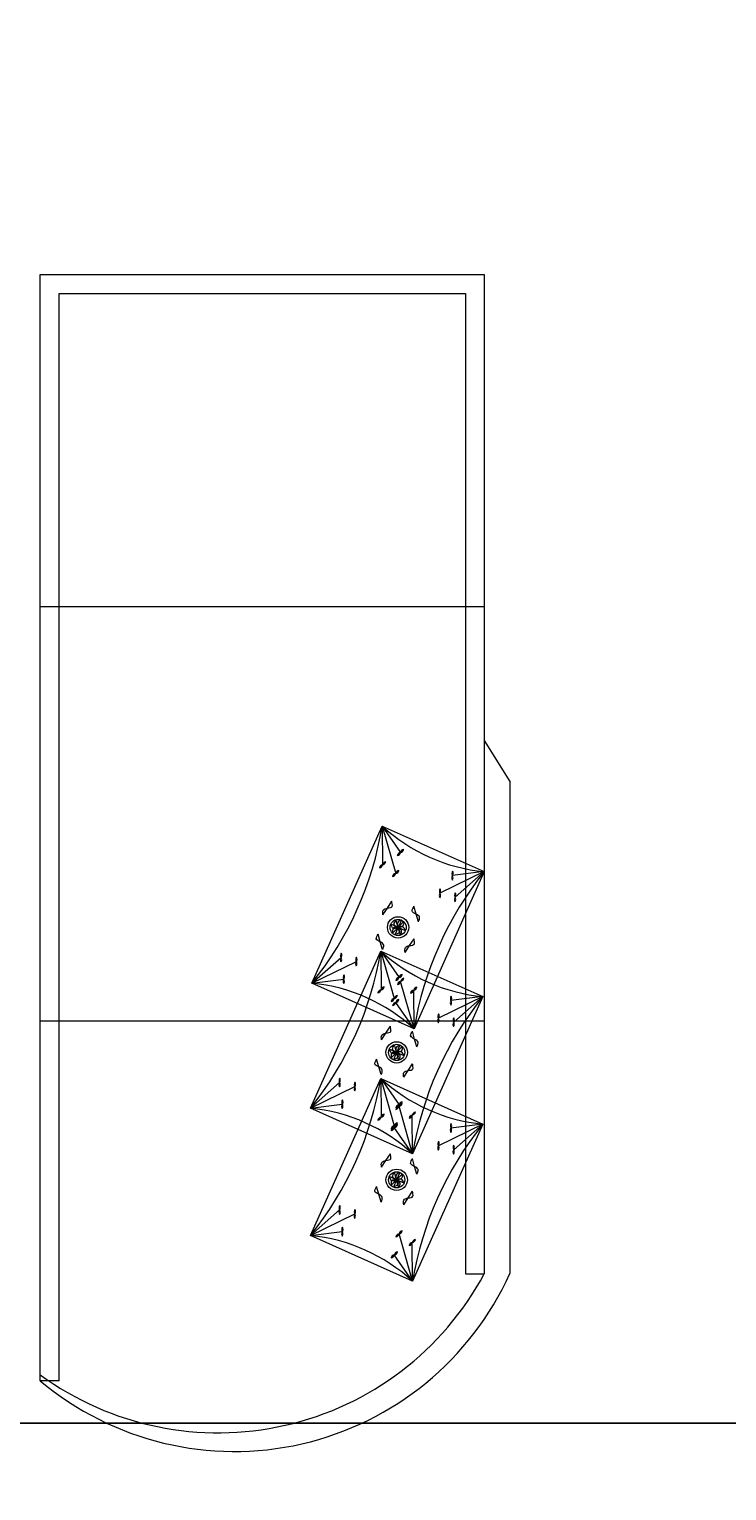
# Model space of a CAD drawing. Units: inches. Extents: x -61 to 1599, y -1316 to 257.
# Tile 12 of 204: x 222 to 259, y -1182 to -1105. Entities that reach past the tile are written whole.
import ezdxf

# ---------------------------------------------------------------- set-up
doc = ezdxf.new("R2010")
doc.units = ezdxf.units.IN
doc.header["$MEASUREMENT"] = 0
doc.layers.add('A-ANNO-DIMS', color=2, linetype='Continuous', lineweight=18)
doc.layers.add('FURNITURE', color=83, linetype='Continuous', lineweight=18)
doc.styles.get("Standard").update_dxf_attribs({"font": 'arial.ttf'})
doc.dimstyles.get("Standard").update_dxf_attribs({"dimtxt": 0.18, "dimasz": 0.18, "dimexe": 0.18, "dimexo": 0.0625, "dimgap": 0.09, "dimtad": 0, "dimtih": 1, "dimtoh": 1, "dimdec": 0, "dimzin": 0, "dimdsep": 46, "dimlunit": 3, "dimtxsty": 'Standard', "dimcen": 0.09, "dimadec": 0, "dimazin": 0, "dimtfac": 1, "dimtdec": 0, "dimtofl": 0, "dimtmove": 0, "dimatfit": 3, "dimfxl": 1, "dimtolj": 1, "dimtzin": 0, "dimarcsym": 0})

# ---------------------------------------------------------------- blocks, each defined once
blk = doc.blocks.new('MASTER-BEDROOM-CONSOLE')
for p, q in [((0, 44.886), (23.587, 44.886)), ((23.587, 37.779), (23.587, 9.438)), ((23.587, 37.779), (24.943, 35.589)), ((24.943, 35.589), (24.943, 9.456)), ((18.162, 33.228), (18.879, 30.704)), ((18.162, 33.228), (19.133, 31.826)), ((18.162, 33.228), (18.181, 31.167)), ((23.587, 30.804), (21.228, 29.654)), ((23.587, 30.804), (21.894, 30.592)), ((23.587, 30.804), (22.038, 29.443)), ((18.203, 28.51), (18.441, 28.869)), ((18.441, 28.869), (18.678, 29.228)), ((19.963, 28.553), (19.841, 28.966)), ((19.008, 27.84), (18.615, 28.016)), ((19.008, 27.84), (18.886, 28.253)), ((19.184, 28.233), (19.008, 27.84)), ((19.309, 28.148), (19.008, 27.84)), ((20.085, 28.141), (19.963, 28.553)), ((18.061, 27.072), (17.939, 27.485)), ((19.008, 27.84), (18.707, 27.533)), ((19.008, 27.84), (18.833, 27.448)), ((19.401, 27.665), (19.008, 27.84)), ((19.13, 27.428), (19.008, 27.84)), ((19.618, 26.876), (19.855, 27.235)), ((18.183, 26.66), (18.061, 27.072)), ((18.084, 26.588), (18.801, 24.064)), ((18.084, 26.588), (19.055, 25.186)), ((18.084, 26.588), (18.103, 24.527)), ((19.38, 26.517), (19.618, 26.876)), ((14.429, 24.877), (15.978, 26.238)), ((14.429, 24.877), (16.788, 26.026)), ((14.429, 24.877), (16.122, 25.089)), ((19.854, 22.452), (19.137, 24.976)), ((19.854, 22.452), (19.835, 24.514)), ((23.509, 24.163), (21.15, 23.014)), ((23.509, 24.163), (21.816, 23.952)), ((23.509, 24.163), (21.96, 22.803)), ((19.854, 22.452), (18.883, 23.854)), ((0, 22.886), (23.587, 22.886)), ((18.362, 22.229), (18.6, 22.588)), ((18.125, 21.87), (18.362, 22.229)), ((19.885, 21.913), (19.763, 22.326)), ((20.007, 21.5), (19.885, 21.913)), ((18.93, 21.2), (18.537, 21.376)), ((18.93, 21.2), (18.629, 20.893)), ((18.93, 21.2), (18.754, 20.808)), ((18.93, 21.2), (18.808, 21.613)), ((19.105, 21.593), (18.93, 21.2)), ((19.23, 21.508), (18.93, 21.2)), ((19.322, 21.025), (18.93, 21.2)), ((19.052, 20.788), (18.93, 21.2)), ((17.983, 20.432), (17.861, 20.845)), ((18.105, 20.02), (17.983, 20.432)), ((19.302, 19.877), (19.54, 20.236)), ((19.54, 20.236), (19.777, 20.595)), ((14.351, 18.237), (15.9, 19.598)), ((18.084, 19.819), (18.801, 17.295)), ((18.084, 19.819), (19.055, 18.417)), ((18.084, 19.819), (18.103, 17.757)), ((14.351, 18.237), (16.71, 19.386)), ((14.351, 18.237), (16.043, 18.448)), ((19.776, 15.812), (19.059, 18.336)), ((19.776, 15.812), (19.757, 17.874)), ((19.776, 15.812), (18.804, 17.214)), ((23.509, 17.394), (21.15, 16.245)), ((23.509, 17.394), (21.816, 17.183)), ((23.509, 17.394), (21.96, 16.033)), ((18.362, 15.459), (18.6, 15.818)), ((19.885, 15.143), (19.763, 15.556)), ((18.125, 15.101), (18.362, 15.459)), ((18.93, 14.431), (18.808, 14.843)), ((19.105, 14.823), (18.93, 14.431)), ((20.007, 14.731), (19.885, 15.143)), ((17.983, 13.663), (17.861, 14.075)), ((18.93, 14.431), (18.537, 14.606)), ((18.93, 14.431), (18.629, 14.123)), ((18.93, 14.431), (18.754, 14.038)), ((19.23, 14.738), (18.93, 14.431)), ((19.322, 14.255), (18.93, 14.431)), ((19.052, 14.018), (18.93, 14.431)), ((18.105, 13.25), (17.983, 13.663)), ((19.302, 13.108), (19.54, 13.466)), ((19.54, 13.466), (19.777, 13.825)), ((14.351, 11.468), (15.9, 12.828)), ((14.351, 11.468), (16.71, 12.617)), ((14.351, 11.468), (16.043, 11.679)), ((19.776, 9.043), (19.059, 11.567)), ((19.776, 9.043), (19.757, 11.104)), ((19.776, 9.043), (18.804, 10.445)), ((22.587, 9.438), (23.587, 9.438)), ((1, 3.748), (0, 3.748))]:
    blk.add_line(p, q)
for points in [[(0, 3.748), (0, 62.524), (23.587, 62.524), (23.587, 9.438)], [(1, 3.748), (1, 61.524), (22.587, 61.524), (22.587, 9.438)]]:
    blk.add_lwpolyline(points)
for points in [[(14.429, 24.877), (18.162, 33.228), (23.587, 30.804), (19.854, 22.452)], [(14.351, 18.237), (18.084, 26.588), (23.509, 24.163), (19.776, 15.812)], [(14.351, 11.468), (18.084, 19.819), (23.509, 17.394), (19.776, 9.043)]]:
    blk.add_lwpolyline(points, close=True)
for centre, radius in [((19.008, 27.84), 0.567), ((19.008, 27.84), 0.567), ((19.008, 27.84), 0.43), ((18.93, 21.2), 0.567), ((18.93, 21.2), 0.567), ((18.93, 21.2), 0.43), ((18.93, 14.431), 0.567), ((18.93, 14.431), 0.567), ((18.93, 14.431), 0.43)]:
    blk.add_circle(centre, radius)
for centre, radius, start, end in [((0.46, 36.131), 17.938, 321.14464, 350.6879), ((24.495, 40.115), 9.356, 227.40134, 264.43121), ((19.095, 32.037), 0.214, 280.21251, 346.40619), ((19.338, 31.78), 0.209, 99.3213, 167.2974), ((18.215, 30.96), 0.209, 99.3213, 167.2974), ((17.973, 31.217), 0.214, 280.21251, 346.40619), ((18.143, 31.378), 0.214, 280.21251, 346.40619), ((18.385, 31.121), 0.209, 99.3213, 167.2974), ((19.167, 31.62), 0.209, 99.3213, 167.2974), ((18.925, 31.877), 0.214, 280.21251, 346.40619), ((18.913, 30.498), 0.209, 99.3213, 167.2974), ((18.67, 30.755), 0.214, 280.21251, 346.40619), ((18.841, 30.915), 0.214, 280.21251, 346.40619), ((19.083, 30.658), 0.209, 99.3213, 167.2974), ((37.556, 19.55), 17.938, 141.14464, 170.6879), ((22.071, 30.471), 0.214, 145.42636, 211.62004), ((22.077, 30.705), 0.214, 145.42636, 211.62004), ((21.718, 30.48), 0.209, 324.53515, 32.51125), ((21.724, 30.714), 0.209, 324.53515, 32.51125), ((21.405, 29.533), 0.214, 145.42636, 211.62004), ((21.411, 29.767), 0.214, 145.42636, 211.62004), ((21.052, 29.542), 0.209, 324.53515, 32.51125), ((21.058, 29.776), 0.209, 324.53515, 32.51125), ((22.221, 29.555), 0.214, 145.42636, 211.62004), ((21.867, 29.564), 0.209, 324.53515, 32.51125), ((22.215, 29.321), 0.214, 145.42636, 211.62004), ((21.861, 29.33), 0.209, 324.53515, 32.51125), ((0.382, 29.491), 17.938, 321.14464, 350.6879), ((16.155, 26.351), 0.209, 144.53515, 212.51125), ((15.802, 26.36), 0.214, 325.42636, 31.62004), ((24.416, 33.475), 9.356, 227.40134, 264.43121), ((16.149, 26.117), 0.209, 144.53515, 212.51125), ((15.796, 26.126), 0.214, 325.42636, 31.62004), ((16.959, 25.905), 0.209, 144.53515, 212.51125), ((16.965, 26.139), 0.209, 144.53515, 212.51125), ((16.605, 25.914), 0.214, 325.42636, 31.62004), ((16.611, 26.148), 0.214, 325.42636, 31.62004), ((13.521, 15.565), 9.356, 47.40134, 84.43121), ((16.292, 24.967), 0.209, 144.53515, 212.51125), ((16.298, 25.201), 0.209, 144.53515, 212.51125), ((15.939, 24.976), 0.214, 325.42636, 31.62004), ((15.945, 25.21), 0.214, 325.42636, 31.62004), ((19.089, 24.98), 0.209, 99.3213, 167.2974), ((18.847, 25.237), 0.214, 280.21251, 346.40619), ((19.175, 24.765), 0.214, 100.21251, 166.40619), ((18.933, 25.022), 0.209, 279.3213, 347.2974), ((19.017, 25.397), 0.214, 280.21251, 346.40619), ((19.259, 25.14), 0.209, 99.3213, 167.2974), ((19.103, 25.183), 0.209, 279.3213, 347.2974), ((19.346, 24.926), 0.214, 100.21251, 166.40619), ((18.137, 24.32), 0.209, 99.3213, 167.2974), ((17.894, 24.577), 0.214, 280.21251, 346.40619), ((18.065, 24.738), 0.214, 280.21251, 346.40619), ((18.307, 24.48), 0.209, 99.3213, 167.2974), ((18.763, 24.275), 0.214, 280.21251, 346.40619), ((19.005, 24.018), 0.209, 99.3213, 167.2974), ((19.873, 24.303), 0.214, 100.21251, 166.40619), ((19.631, 24.56), 0.209, 279.3213, 347.2974), ((37.478, 12.91), 17.938, 141.14464, 170.6879), ((19.801, 24.721), 0.209, 279.3213, 347.2974), ((20.043, 24.464), 0.214, 100.21251, 166.40619), ((21.999, 24.065), 0.214, 145.42636, 211.62004), ((21.646, 24.074), 0.209, 324.53515, 32.51125), ((18.834, 23.858), 0.209, 99.3213, 167.2974), ((18.592, 24.115), 0.214, 280.21251, 346.40619), ((18.921, 23.643), 0.214, 100.21251, 166.40619), ((18.678, 23.9), 0.209, 279.3213, 347.2974), ((18.849, 24.061), 0.209, 279.3213, 347.2974), ((19.091, 23.804), 0.214, 100.21251, 166.40619), ((21.993, 23.83), 0.214, 145.42636, 211.62004), ((21.64, 23.84), 0.209, 324.53515, 32.51125), ((21.326, 22.892), 0.214, 145.42636, 211.62004), ((21.332, 23.127), 0.214, 145.42636, 211.62004), ((20.973, 22.902), 0.209, 324.53515, 32.51125), ((20.979, 23.136), 0.209, 324.53515, 32.51125), ((22.136, 22.681), 0.214, 145.42636, 211.62004), ((22.142, 22.915), 0.214, 145.42636, 211.62004), ((21.783, 22.69), 0.209, 324.53515, 32.51125), ((21.789, 22.924), 0.209, 324.53515, 32.51125), ((0.382, 22.721), 17.938, 321.14464, 350.6879), ((16.07, 19.476), 0.209, 144.53515, 212.51125), ((16.076, 19.711), 0.209, 144.53515, 212.51125), ((15.717, 19.486), 0.214, 325.42636, 31.62004), ((15.723, 19.72), 0.214, 325.42636, 31.62004), ((16.886, 19.499), 0.209, 144.53515, 212.51125), ((16.533, 19.508), 0.214, 325.42636, 31.62004), ((24.416, 26.706), 9.356, 227.40134, 264.43121), ((16.22, 18.561), 0.209, 144.53515, 212.51125), ((15.867, 18.57), 0.214, 325.42636, 31.62004), ((16.88, 19.265), 0.209, 144.53515, 212.51125), ((16.527, 19.274), 0.214, 325.42636, 31.62004), ((13.443, 8.925), 9.356, 47.40134, 84.43121), ((16.214, 18.327), 0.209, 144.53515, 212.51125), ((15.861, 18.336), 0.214, 325.42636, 31.62004), ((18.065, 17.968), 0.214, 280.21251, 346.40619), ((18.307, 17.711), 0.209, 99.3213, 167.2974), ((19.089, 18.21), 0.209, 99.3213, 167.2974), ((18.847, 18.467), 0.214, 280.21251, 346.40619), ((19.097, 18.125), 0.214, 100.21251, 166.40619), ((18.855, 18.382), 0.209, 279.3213, 347.2974), ((19.017, 18.628), 0.214, 280.21251, 346.40619), ((19.259, 18.371), 0.209, 99.3213, 167.2974), ((19.025, 18.543), 0.209, 279.3213, 347.2974), ((19.267, 18.286), 0.214, 100.21251, 166.40619), ((19.795, 17.663), 0.214, 100.21251, 166.40619), ((19.552, 17.92), 0.209, 279.3213, 347.2974), ((19.723, 18.081), 0.209, 279.3213, 347.2974), ((19.965, 17.824), 0.214, 100.21251, 166.40619), ((18.137, 17.55), 0.209, 99.3213, 167.2974), ((17.894, 17.807), 0.214, 280.21251, 346.40619), ((18.834, 17.088), 0.209, 99.3213, 167.2974), ((18.592, 17.345), 0.214, 280.21251, 346.40619), ((18.842, 17.003), 0.214, 100.21251, 166.40619), ((18.6, 17.26), 0.209, 279.3213, 347.2974), ((18.763, 17.506), 0.214, 280.21251, 346.40619), ((19.005, 17.249), 0.209, 99.3213, 167.2974), ((18.771, 17.421), 0.209, 279.3213, 347.2974), ((19.013, 17.164), 0.214, 100.21251, 166.40619), ((37.478, 6.14), 17.938, 141.14464, 170.6879), ((21.993, 17.061), 0.214, 145.42636, 211.62004), ((21.999, 17.295), 0.214, 145.42636, 211.62004), ((21.64, 17.07), 0.209, 324.53515, 32.51125), ((21.646, 17.304), 0.209, 324.53515, 32.51125), ((21.332, 16.357), 0.214, 145.42636, 211.62004), ((20.979, 16.366), 0.209, 324.53515, 32.51125), ((21.326, 16.123), 0.214, 145.42636, 211.62004), ((20.973, 16.132), 0.209, 324.53515, 32.51125), ((22.136, 15.911), 0.214, 145.42636, 211.62004), ((22.142, 16.145), 0.214, 145.42636, 211.62004), ((21.783, 15.92), 0.209, 324.53515, 32.51125), ((21.789, 16.155), 0.209, 324.53515, 32.51125), ((16.07, 12.707), 0.209, 144.53515, 212.51125), ((16.076, 12.941), 0.209, 144.53515, 212.51125), ((15.717, 12.716), 0.214, 325.42636, 31.62004), ((15.723, 12.95), 0.214, 325.42636, 31.62004), ((16.88, 12.495), 0.209, 144.53515, 212.51125), ((16.886, 12.729), 0.209, 144.53515, 212.51125), ((16.527, 12.504), 0.214, 325.42636, 31.62004), ((16.533, 12.739), 0.214, 325.42636, 31.62004), ((16.214, 11.557), 0.209, 144.53515, 212.51125), ((16.22, 11.791), 0.209, 144.53515, 212.51125), ((15.861, 11.566), 0.214, 325.42636, 31.62004), ((15.867, 11.801), 0.214, 325.42636, 31.62004), ((19.025, 11.773), 0.209, 279.3213, 347.2974), ((19.267, 11.516), 0.214, 100.21251, 166.40619), ((13.443, 2.156), 9.356, 47.40134, 84.43121), ((19.097, 11.356), 0.214, 100.21251, 166.40619), ((18.855, 11.613), 0.209, 279.3213, 347.2974), ((19.795, 10.893), 0.214, 100.21251, 166.40619), ((19.552, 11.151), 0.209, 279.3213, 347.2974), ((19.723, 11.311), 0.209, 279.3213, 347.2974), ((19.965, 11.054), 0.214, 100.21251, 166.40619), ((18.842, 10.234), 0.214, 100.21251, 166.40619), ((18.6, 10.491), 0.209, 279.3213, 347.2974), ((18.771, 10.651), 0.209, 279.3213, 347.2974), ((19.013, 10.394), 0.214, 100.21251, 166.40619), ((10.308, 16.053), 16.053, 230.04489, 335.73444), ((9.449, 17.042), 16.053, 233.93821, 331.72641)]:
    blk.add_arc(centre, radius, start, end)
for points in [[(18.203, 28.51), (18.191, 28.604), (18.167, 28.791), (18.438, 28.884), (18.778, 28.897), (18.67, 29.157), (18.678, 29.228)], [(20.085, 28.141), (20.124, 28.226), (20.202, 28.398), (19.97, 28.566), (19.649, 28.679), (19.829, 28.896), (19.841, 28.966)], [(19.401, 27.665), (19.361, 27.75), (19.281, 27.921), (19.003, 27.854), (18.708, 27.683), (18.66, 27.961), (18.615, 28.016)], [(19.309, 28.148), (19.303, 28.054), (19.292, 27.866), (19.008, 27.825), (18.671, 27.876), (18.729, 27.6), (18.707, 27.533)], [(19.13, 27.428), (19.169, 27.514), (19.247, 27.685), (19.015, 27.854), (18.694, 27.966), (18.873, 28.183), (18.886, 28.253)], [(19.184, 28.233), (19.098, 28.193), (18.927, 28.113), (18.994, 27.835), (19.165, 27.54), (18.888, 27.492), (18.833, 27.448)], [(18.183, 26.66), (18.222, 26.746), (18.3, 26.917), (18.069, 27.086), (17.747, 27.198), (17.927, 27.415), (17.939, 27.485)], [(19.38, 26.517), (19.368, 26.611), (19.344, 26.798), (19.615, 26.891), (19.955, 26.904), (19.847, 27.164), (19.855, 27.235)], [(18.125, 21.87), (18.113, 21.964), (18.089, 22.151), (18.359, 22.244), (18.7, 22.257), (18.592, 22.517), (18.6, 22.588)], [(20.007, 21.5), (20.046, 21.586), (20.124, 21.758), (19.892, 21.926), (19.571, 22.039), (19.75, 22.256), (19.763, 22.326)], [(19.322, 21.025), (19.283, 21.11), (19.203, 21.281), (18.924, 21.214), (18.63, 21.043), (18.582, 21.321), (18.537, 21.376)], [(19.23, 21.508), (19.225, 21.414), (19.213, 21.226), (18.93, 21.185), (18.593, 21.236), (18.651, 20.96), (18.629, 20.893)], [(19.052, 20.788), (19.091, 20.874), (19.169, 21.045), (18.937, 21.214), (18.615, 21.326), (18.795, 21.543), (18.808, 21.613)], [(19.105, 21.593), (19.02, 21.553), (18.849, 21.473), (18.916, 21.195), (19.087, 20.9), (18.809, 20.852), (18.754, 20.808)], [(18.105, 20.02), (18.144, 20.105), (18.222, 20.277), (17.99, 20.445), (17.669, 20.558), (17.848, 20.775), (17.861, 20.845)], [(19.302, 19.877), (19.29, 19.971), (19.266, 20.158), (19.537, 20.251), (19.877, 20.264), (19.769, 20.524), (19.777, 20.595)], [(18.125, 15.101), (18.113, 15.194), (18.089, 15.381), (18.359, 15.474), (18.7, 15.488), (18.592, 15.748), (18.6, 15.818)], [(20.007, 14.731), (20.046, 14.817), (20.124, 14.988), (19.892, 15.157), (19.571, 15.269), (19.75, 15.486), (19.763, 15.556)], [(19.052, 14.018), (19.091, 14.104), (19.169, 14.276), (18.937, 14.444), (18.615, 14.557), (18.795, 14.773), (18.808, 14.843)], [(19.105, 14.823), (19.02, 14.784), (18.849, 14.704), (18.916, 14.425), (19.087, 14.131), (18.809, 14.083), (18.754, 14.038)], [(18.105, 13.25), (18.144, 13.336), (18.222, 13.508), (17.99, 13.676), (17.669, 13.788), (17.848, 14.005), (17.861, 14.075)], [(19.322, 14.255), (19.283, 14.341), (19.203, 14.511), (18.924, 14.445), (18.63, 14.274), (18.582, 14.551), (18.537, 14.606)], [(19.23, 14.738), (19.225, 14.644), (19.213, 14.456), (18.93, 14.416), (18.593, 14.466), (18.651, 14.191), (18.629, 14.123)], [(19.302, 13.108), (19.29, 13.201), (19.266, 13.388), (19.537, 13.481), (19.877, 13.495), (19.769, 13.755), (19.777, 13.825)]]:
    blk.add_open_spline(points, degree=3, knots=[0, 0, 0, 0, 0.249187, 0.498374, 0.766554, 1.034734, 1.034734, 1.034734, 1.034734])
blk = doc.blocks.new('*D687')
at = {"layer": 'A-ANNO-DIMS', "color": 0, "lineweight": -2, "transparency": 16777216}
for p, q in [((289.418, 181.677), (-61.077, 181.677)), ((-60.897, 181.497), (-60.897, -528.952)), ((-60.897, -1239.765), (-60.897, -529.316)), ((319.64, -1239.945), (-61.077, -1239.945))]:
    blk.add_line(p, q, dxfattribs=at)
at = {"layer": 'A-ANNO-DIMS', "color": 0, "transparency": 16777216}
for points in [[(-60.927, 181.497), (-60.867, 181.497), (-60.897, 181.677)], [(-60.927, -1239.765), (-60.867, -1239.765), (-60.897, -1239.945)]]:
    blk.add_solid(points, dxfattribs=at)
at = {"layer": 'DEFPOINTS', "color": 0, "transparency": 16777216}
for p in [(289.481, 181.677), (-60.897, -1239.945), (319.703, -1239.945)]:
    blk.add_point(p, dxfattribs=at)
at = {"layer": 'A-ANNO-DIMS', "color": 0, "transparency": 16777216, "insert": (-60.897, -529.134), "char_height": 0.18, "attachment_point": 5}
blk.add_mtext('\\A1;1421.6', dxfattribs=at)
blk = doc.blocks.new('*D696')
at = {"layer": 'A-ANNO-DIMS', "color": 0, "lineweight": -2, "transparency": 16777216}
for p, q in [((690.64, -873.169), (-61.077, -873.169)), ((-60.897, -873.349), (-60.897, -1025.799)), ((-60.897, -1178.613), (-60.897, -1026.163)), ((690.64, -1178.793), (-61.077, -1178.793))]:
    blk.add_line(p, q, dxfattribs=at)
at = {"layer": 'A-ANNO-DIMS', "color": 0, "transparency": 16777216}
for points in [[(-60.927, -873.349), (-60.867, -873.349), (-60.897, -873.169)], [(-60.927, -1178.613), (-60.867, -1178.613), (-60.897, -1178.793)]]:
    blk.add_solid(points, dxfattribs=at)
at = {"layer": 'DEFPOINTS', "color": 0, "transparency": 16777216}
for p in [(-60.897, -873.169), (690.703, -873.169), (690.703, -1178.793)]:
    blk.add_point(p, dxfattribs=at)
at = {"layer": 'A-ANNO-DIMS', "color": 0, "transparency": 16777216, "insert": (-60.897, -1025.981), "char_height": 0.18, "attachment_point": 5}
blk.add_mtext('\\A1;305.6', dxfattribs=at)

msp = doc.modelspace()

# ---------------------------------------------------------------- block references
at = {"layer": 'FURNITURE'}
msp.add_blockref('MASTER-BEDROOM-CONSOLE', (222.602, -1180.2887), dxfattribs=at)

# ---------------------------------------------------------------- dimensions: what is measured, and where the dimension line sits
at = {"layer": 'A-ANNO-DIMS'}
for base, p1, p2, picture, middle in [((-60.8972, -1239.9446), (289.4807, 181.6771), (319.7028, -1239.9446), '*D687', (-60.8972, -529.1337)), ((-60.8972, -873.169), (690.7028, -1178.7933), (690.7028, -873.169), '*D696', (-60.8972, -1025.9812))]:
    dim = msp.add_linear_dim(base=base, p1=p1, p2=p2, angle=90, dimstyle='Standard', override={"dimdec": 1, "dimlfac": 1, "dimrnd": 0, "dimzin": 0, "dimdsep": 46, "dimlunit": 2}, dxfattribs=at)
    dim.commit()
    dim.dimension.update_dxf_attribs({"geometry": picture, "text_midpoint": middle})

doc.saveas('drawing.dxf')
